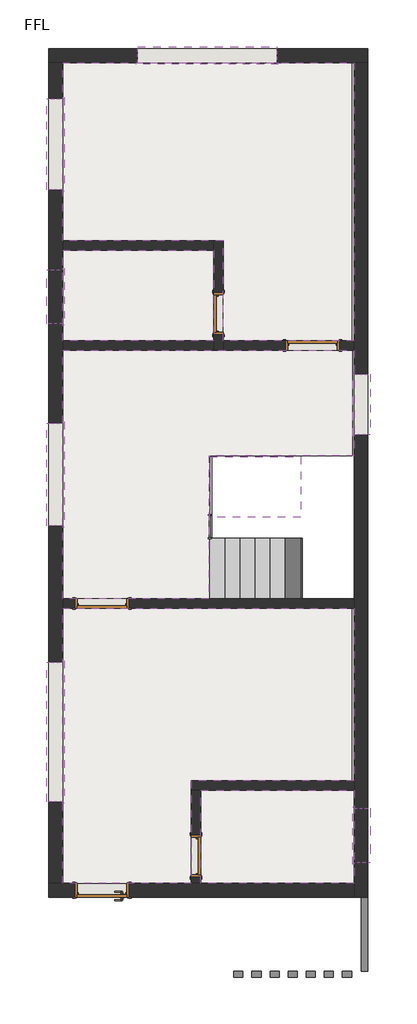
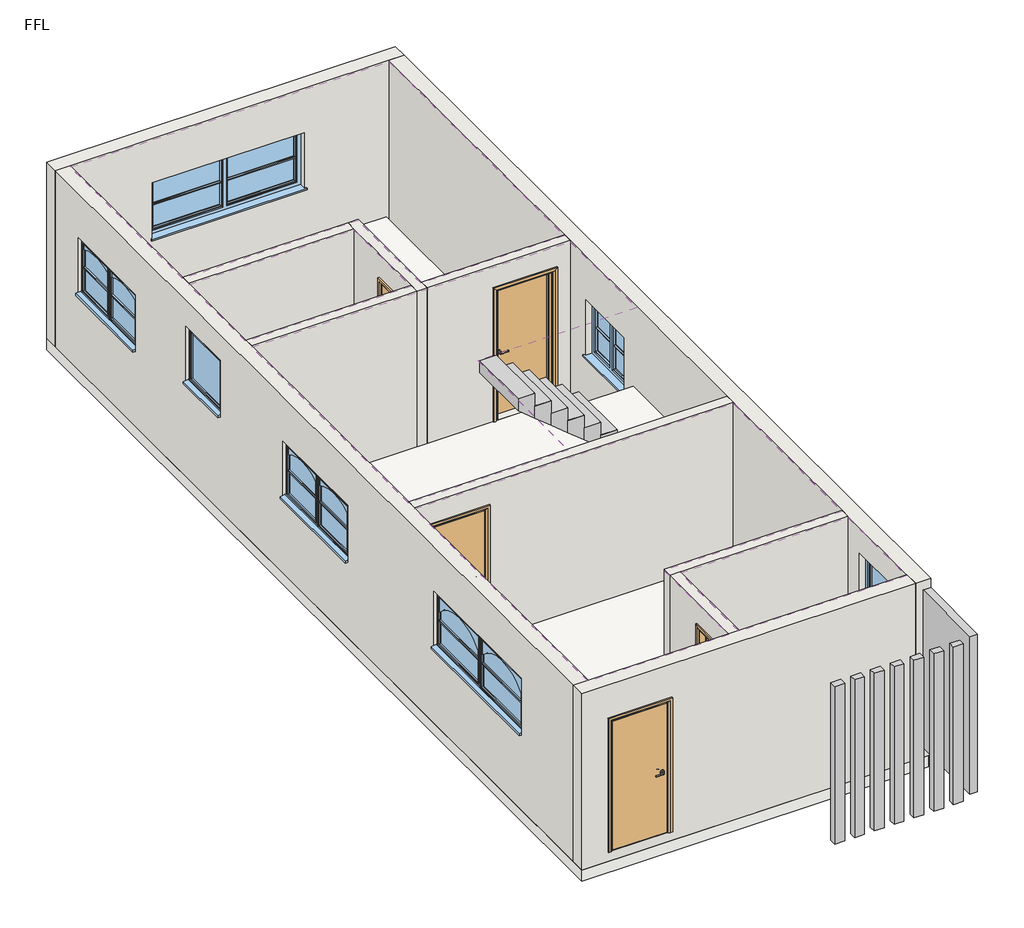
# One storey, incomplete: 11 walls, 7 windows, 6 slabs, 5 coverings, 5 doors, 2 furniture elements, 2 stair flights, 1 railing.
"""IFC4 building model written with IfcOpenShell, lengths in millimetres."""

from ifc_helpers import new_model, si_unit, point, frame, origin, place, context, project, spatial, polyline, ellipse_curve, trimmed, outline, extrude, faceted_brep, transform, mapped, element, save
from ifc_brep_helpers import plane_surface, extruded_surface, advanced_brep
from components import doors_intsgl_1_0_7m_00cad461, doors_intsgl_1_0_7m_20e7f540, doors_intsgl_1_0_9m_7aac3a70, doors_intsgl_1_0_9m_a04e9bb1, casework_1_casework_1_07494d98, casework_3_casework_3_48862e2f, windows_dbl_swept_head_1_m_37dff1ae, windows_dbl_swept_head_1_5_m_7eee1f0c, windows_dbl_swept_head_1_7_m_3b36615c, windows_dbl_swept_head_2_3_m_acbf59cb, windows_sgl_plain_0_9_m_ad1c2cf7

model = new_model("IFC4")

# Units and contexts
model_context = context("Model", 3, world=origin())
ifc_project = project(units=[si_unit("LENGTHUNIT", "METRE", prefix="MILLI")], contexts=[model_context])

# Site, building, storey
site = spatial("IfcSite", under=ifc_project)
building = spatial("IfcBuilding", under=site)
storey = spatial("IfcBuildingStorey", under=building, Name="FFL", Elevation=3000.0)

# Coverings
placement = place(None, origin())
element("IfcCovering", 1, ObjectType="Plain", at=placement, inside=storey, context=model_context, shape_type="SweptSolid", body=[
    extrude(outline(polyline([(-21137.0794706, 13667.7258404), (-16316.1794706, 13667.7258404), (-16316.1794706, 9066.7973913), (-18484.6794706, 9066.7973913), (-18484.6794706, 10719.1973913), (-21137.0794706, 10719.1973913), (-21137.0794706, 13667.7258404)])), frame((0.0, 0.0, 5800.0), z_axis=(0.0, 0.0, 1.0), x_axis=(1.0, 0.0, 0.0)), (0.0, 0.0, 1.0), 57.0),
])
element("IfcCovering", 2, ObjectType="Plain", at=placement, inside=storey, context=model_context, shape_type="SweptSolid", body=[
    extrude(outline(polyline([(-21137.0794706, 9066.7973913), (-21137.0794706, 10566.7973913), (-18637.0794706, 10566.7973913), (-18637.0794706, 9066.7973913), (-21137.0794706, 9066.7973913)])), frame((0.0, 0.0, 5800.0), z_axis=(0.0, 0.0, 1.0), x_axis=(1.0, 0.0, 0.0)), (0.0, 0.0, 1.0), 57.0),
])
element("IfcCovering", 3, ObjectType="Plain", at=placement, inside=storey, context=model_context, shape_type="SweptSolid", body=[
    extrude(outline(polyline([(-16316.1794706, 8914.3973913), (-16316.1794706, 7168.7350753), (-18722.2278737, 7168.7350753), (-18722.2278737, 4801.1258404), (-21137.0794706, 4801.1258404), (-21137.0794706, 8914.3973913), (-18560.8794706, 8914.3973913), (-16316.1794706, 8914.3973913)])), frame((0.0, 0.0, 5800.0), z_axis=(0.0, 0.0, 1.0), x_axis=(1.0, 0.0, 0.0)), (0.0, 0.0, 1.0), 57.0),
])
element("IfcCovering", 4, ObjectType="Plain", at=placement, inside=storey, context=model_context, shape_type="SweptSolid", body=[
    extrude(outline(polyline([(-16316.1794706, 4648.7258404), (-16316.1794706, 1791.1258404), (-19006.6794706, 1791.1258404), (-19006.6794706, 96.3258404), (-21137.0794706, 96.3258404), (-21137.0794706, 4648.7258404), (-16316.1794706, 4648.7258404)])), frame((0.0, 0.0, 5800.0), z_axis=(0.0, 0.0, 1.0), x_axis=(1.0, 0.0, 0.0)), (0.0, 0.0, 1.0), 57.0),
])
element("IfcCovering", 5, ObjectType="Plain", at=placement, inside=storey, context=model_context, shape_type="SweptSolid", body=[
    extrude(outline(polyline([(-18854.2794706, 1638.7258404), (-16316.1794706, 1638.7258404), (-16316.1794706, 96.3258404), (-18854.2794706, 96.3258404), (-18854.2794706, 1638.7258404)])), frame((0.0, 0.0, 5800.0), z_axis=(0.0, 0.0, 1.0), x_axis=(1.0, 0.0, 0.0)), (0.0, 0.0, 1.0), 57.0),
])

# Doors
doors_intsgl_1_0_7m_shape = doors_intsgl_1_0_7m_00cad461(model_context)
element("IfcDoor", 6, ObjectType="Doors_IntSgl_1 : 0.7M", at=placement, inside=storey, context=model_context, shape_type="MappedRepresentation", body=[
    mapped(doors_intsgl_1_0_7m_shape, transform((-18930.4794706, 546.3258404, 3330.0), x_axis=(0.0, -1.0, 0.0), y_axis=(1.0, 0.0, 0.0), z_axis=(0.0, 0.0, 1.0))),
])
doors_intsgl_1_0_7m_2_shape = doors_intsgl_1_0_7m_20e7f540(model_context)
element("IfcDoor", 7, ObjectType="Doors_IntSgl_1 : 0.7M", at=placement, inside=storey, context=model_context, shape_type="MappedRepresentation", body=[
    mapped(doors_intsgl_1_0_7m_2_shape, transform((-18560.8794706, 9516.7973913, 3300.0), x_axis=(0.0, -1.0, 0.0), y_axis=(1.0, 0.0, 0.0), z_axis=(0.0, 0.0, 1.0))),
])
doors_intsgl_1_0_9m_shape = doors_intsgl_1_0_9m_7aac3a70(model_context)
element("IfcDoor", 8, ObjectType="Doors_IntSgl_1 : 0.9M", at=placement, inside=storey, context=model_context, shape_type="MappedRepresentation", body=[
    mapped(doors_intsgl_1_0_9m_shape, transform((-17004.2794706, 8990.5973913, 3330.0), x_axis=(1.0, 0.0, 0.0), y_axis=(0.0, 1.0, 0.0), z_axis=(0.0, 0.0, 1.0))),
])
element("IfcDoor", 9, ObjectType="Doors_IntSgl_1 : 0.9M", at=placement, inside=storey, context=model_context, shape_type="MappedRepresentation", body=[
    mapped(doors_intsgl_1_0_9m_shape, transform((-20487.0794706, 4724.9258404, 3330.0), x_axis=(-1.0, 0.0, 0.0), y_axis=(0.0, -1.0, 0.0), z_axis=(0.0, 0.0, 1.0))),
])
doors_intsgl_1_0_9m_2_shape = doors_intsgl_1_0_9m_a04e9bb1(model_context)
element("IfcDoor", 10, ObjectType="Doors_IntSgl_1 : 0.9M", at=placement, inside=storey, context=model_context, shape_type="MappedRepresentation", body=[
    mapped(doors_intsgl_1_0_9m_2_shape, transform((-20487.0794706, -17.9741596, 3150.0), x_axis=(-1.0, 0.0, 0.0), y_axis=(0.0, -1.0, 0.0), z_axis=(0.0, 0.0, 1.0))),
])

# Furniture
casework_1_casework_1_shape = casework_1_casework_1_07494d98(model_context)
element("IfcFurniture", 11, ObjectType="Casework 1 : Casework 1", at=placement, inside=storey, context=model_context, shape_type="MappedRepresentation", body=[
    mapped(casework_1_casework_1_shape, transform((0.0, 0.0, 0.0), x_axis=(1.0, 0.0, 0.0), y_axis=(0.0, 1.0, 0.0), z_axis=(0.0, 0.0, 1.0))),
])
casework_3_casework_3_shape = casework_3_casework_3_48862e2f(model_context)
element("IfcFurniture", 12, ObjectType="Casework 3 : Casework 3", at=placement, inside=storey, context=model_context, shape_type="MappedRepresentation", body=[
    mapped(casework_3_casework_3_shape, transform((0.0, 0.0, 0.0), x_axis=(1.0, 0.0, 0.0), y_axis=(0.0, 1.0, 0.0), z_axis=(0.0, 0.0, 1.0))),
])

# Railing
element("IfcRailing", 13, ObjectType="Glass_Panel-Bottom_Fill", at=placement, inside=storey, context=model_context, shape_type="SolidModel", body=[
    advanced_brep(
    [(-18745.2702358, 5800.7258404, 4230.0), (-18665.2702358, 5800.7258404, 4230.0), (-18745.2702358, 6188.9258404, 4230.0), (-18665.2702358, 6188.9258404, 4230.0)],
    [
        (0, 1, ellipse_curve(frame((-18705.2702358, 5800.7258404, 4230.0), z_axis=(0.0, -1.0, 0.0), x_axis=(1.0, 0.0, 0.0)), 40.0, 30.0)),
        (1, 0, ellipse_curve(frame((-18705.2702358, 5800.7258404, 4230.0), z_axis=(0.0, -1.0, 0.0), x_axis=(1.0, 0.0, 0.0)), 40.0, 30.0)),
        (2, 3, ellipse_curve(frame((-18705.2702358, 6188.9258404, 4230.0), z_axis=(0.0, 1.0, 0.0), x_axis=(1.0, 0.0, 0.0)), 40.0, 30.0)),
        (3, 2, ellipse_curve(frame((-18705.2702358, 6188.9258404, 4230.0), z_axis=(0.0, 1.0, 0.0), x_axis=(1.0, 0.0, 0.0)), 40.0, 30.0)),
        (0, 2),
        (3, 1),
    ],
    [
        plane_surface(frame((-18705.2702358, 5800.7258404, 4230.0), z_axis=(0.0, -1.0, 0.0), x_axis=(0.0, 0.0, 1.0))),
        plane_surface(frame((-18705.2702358, 6188.9258404, 4230.0), z_axis=(0.0, 1.0, 0.0), x_axis=(0.0, 0.0, 1.0))),
        extruded_surface(trimmed(ellipse_curve(frame((-18705.2702358, 6188.9258404, 4230.0), z_axis=(0.0, -1.0, 0.0), x_axis=(1.0, 0.0, 0.0)), 40.0, 30.0), [point((-18745.2702358, 6188.9258404, 4230.0))], [point((-18665.2702358, 6188.9258404, 4230.0))], True, "CARTESIAN"), (0.0, -388.1999999999998, 0.0), 388.1999999999998),
        extruded_surface(trimmed(ellipse_curve(frame((-18705.2702358, 6188.9258404, 4230.0), z_axis=(0.0, -1.0, 0.0), x_axis=(1.0, 0.0, 0.0)), 40.0, 30.0), [point((-18665.2702358, 6188.9258404, 4230.0))], [point((-18745.2702358, 6188.9258404, 4230.0))], True, "CARTESIAN"), (0.0, -388.1999999999998, 0.0), 388.1999999999998),
    ],
    [
        (0, [[1, 2]]),
        (1, [[3, 4]]),
        (2, [[-1, 5, -4, 6]]),
        (3, [[-2, -6, -3, -5]]),
    ],
),
    extrude(outline(polyline([(-18695.8794706, 5800.7258404), (-18715.8794706, 5800.7258404), (-18715.8794706, 6188.9258404), (-18695.8794706, 6188.9258404), (-18695.8794706, 5800.7258404)])), frame((0.0, 0.0, 4110.0), z_axis=(0.0, 0.0, 1.0), x_axis=(1.0, 0.0, 0.0)), (0.0, 0.0, 1.0), 20.0),
    extrude(outline(polyline([(-18695.8794706, 5800.7258404), (-18715.8794706, 5800.7258404), (-18715.8794706, 6188.9258404), (-18695.8794706, 6188.9258404), (-18695.8794706, 5800.7258404)])), frame((0.0, 0.0, 4010.0), z_axis=(0.0, 0.0, 1.0), x_axis=(1.0, 0.0, 0.0)), (0.0, 0.0, 1.0), 20.0),
    extrude(outline(polyline([(-18730.8794706, 6180.9258404), (-18730.8794706, 6192.9258404), (-18680.8794706, 6192.9258404), (-18680.8794706, 6180.9258404), (-18730.8794706, 6180.9258404)])), frame((0.0, 0.0, 3330.0), z_axis=(0.0, 0.0, 1.0), x_axis=(1.0, 0.0, 0.0)), (0.0, 0.0, 1.0), 870.0),
    extrude(outline(polyline([(-18730.8794706, 5796.7258404), (-18730.8794706, 5808.7258404), (-18680.8794706, 5808.7258404), (-18680.8794706, 5796.7258404), (-18730.8794706, 5796.7258404)])), frame((0.0, 0.0, 3330.0), z_axis=(0.0, 0.0, 1.0), x_axis=(1.0, 0.0, 0.0)), (0.0, 0.0, 1.0), 870.0),
])

# Slabs
element("IfcSlab", 14, ObjectType="200mm_Thickness", at=placement, inside=storey, context=model_context, shape_type="SolidModel", body=[
    faceted_brep([(-17201.8794706, 5801.1258404, 4574.0), (-17201.8794706, 4801.1258404, 4574.0), (-16959.9361063, 4801.1258404, 4574.0), (-16381.8794706, 4801.1258404, 4574.0), (-16381.8794706, 7153.5258404, 4574.0), (-17193.8228349, 7153.5258404, 4574.0), (-17201.8794706, 7153.5258404, 4574.0), (-17201.8794706, 6153.5258404, 4574.0), (-17201.8794706, 5801.1258404, 4374.0), (-17201.8794706, 5801.1258404, 4370.4285714), (-17201.8794706, 5801.1258404, 4176.9889748), (-17201.8794706, 4801.1258404, 4176.9889748), (-17201.8794706, 4801.1258404, 4370.4285714), (-16959.9361063, 4801.1258404, 4374.0), (-16381.8794706, 4801.1258404, 4374.0), (-16381.8794706, 7153.5258404, 4374.0), (-17193.8228349, 7153.5258404, 4374.0), (-17201.8794706, 7153.5258404, 4380.5604034), (-17201.8794706, 6153.5258404, 4380.5604034), (-17201.8794706, 6153.5258404, 4374.0), (-17193.8228349, 6153.5258404, 4374.0), (-16959.9361063, 5801.1258404, 4374.0)], [[[0, 1, 2, 3, 4, 5, 6, 7]], [[1, 0, 8, 9, 10, 11, 12]], [[1, 12, 11, 13, 14, 3, 2]], [[4, 3, 14, 15]], [[4, 15, 16, 17, 6, 5]], [[7, 6, 17, 18]], [[0, 7, 18, 19, 8]], [[19, 20, 16, 15, 14, 13, 21, 8]], [[20, 19, 18]], [[21, 13, 11, 10]], [[8, 21, 10, 9]], [[16, 20, 18, 17]]]),
    extrude(outline(polyline([(-17201.8794706, 5801.1258404), (-17201.8794706, 6153.5258404), (-17201.8794706, 7153.5258404), (-16381.8794706, 7153.5258404), (-16381.8794706, 4801.1258404), (-17201.8794706, 4801.1258404), (-17201.8794706, 5801.1258404)])), frame((0.0, 0.0, 4574.0), z_axis=(0.0, 0.0, 1.0), x_axis=(1.0, 0.0, 0.0)), (0.0, 0.0, 1.0), 1.0),
])
element("IfcSlab", 15, ObjectType="BEDROOM FLOOR", at=placement, inside=storey, context=model_context, shape_type="SweptSolid", body=[
    extrude(outline(polyline([(-21137.0794706, 13667.7258404), (-16354.2794706, 13667.7258404), (-16354.2794706, 9066.7973913), (-18484.6794706, 9066.7973913), (-18484.6794706, 10719.1973913), (-21137.0794706, 10719.1973913), (-21137.0794706, 13667.7258404)])), frame((0.0, 0.0, 3180.0), z_axis=(0.0, 0.0, 1.0), x_axis=(1.0, 0.0, 0.0)), (0.0, 0.0, 1.0), 150.0),
    extrude(outline(polyline([(-19006.6794706, 96.3258404), (-21137.0794706, 96.3258404), (-21137.0794706, 4648.7258404), (-18589.4794706, 4648.7258404), (-16354.2794706, 4648.7258404), (-16354.2794706, 1791.1258404), (-19006.6794706, 1791.1258404), (-19006.6794706, 96.3258404)])), frame((0.0, 0.0, 3180.0), z_axis=(0.0, 0.0, 1.0), x_axis=(1.0, 0.0, 0.0)), (0.0, 0.0, 1.0), 150.0),
])
element("IfcSlab", 16, ObjectType="FAMILY LOUNGE", at=placement, inside=storey, context=model_context, shape_type="SweptSolid", body=[
    extrude(outline(polyline([(-18701.8794706, 4801.1258404), (-21137.0794706, 4801.1258404), (-21137.0794706, 8914.3973913), (-16351.8794706, 8914.3973913), (-16351.8794706, 7168.7613597), (-18701.8794706, 7168.7613597), (-18701.8794706, 4801.1258404)])), frame((0.0, 0.0, 3180.0), z_axis=(0.0, 0.0, 1.0), x_axis=(1.0, 0.0, 0.0)), (0.0, 0.0, 1.0), 150.0),
])
element("IfcSlab", 17, ObjectType="SLAB", at=placement, inside=storey, context=model_context, shape_type="SweptSolid", body=[
    extrude(outline(polyline([(-16125.6794706, 13896.3258404), (-16125.6794706, -132.2741596), (-21365.6794706, -132.2741596), (-21365.6794706, 13896.3258404), (-16125.6794706, 13896.3258404)]), holes=[polyline([(-16316.1794706, 7168.7350753), (-18663.7794706, 7168.7350753), (-18663.7794706, 4801.1258404), (-16316.1794706, 4801.1258404), (-16316.1794706, 7168.7350753)])]), frame((0.0, 0.0, 2820.0), z_axis=(0.0, 0.0, 1.0), x_axis=(1.0, 0.0, 0.0)), (0.0, 0.0, 1.0), 180.0),
])
element("IfcSlab", 18, ObjectType="TOILET FLOOR", at=placement, inside=storey, context=model_context, shape_type="SweptSolid", body=[
    extrude(outline(polyline([(-18637.0794706, 10566.7973913), (-18637.0794706, 9066.7973913), (-21137.0794706, 9066.7973913), (-21137.0794706, 10566.7973913), (-18637.0794706, 10566.7973913)])), frame((0.0, 0.0, 3000.0), z_axis=(0.0, 0.0, 1.0), x_axis=(1.0, 0.0, 0.0)), (0.0, 0.0, 1.0), 300.0),
])
element("IfcSlab", 19, ObjectType="TOILET FLOOR", at=placement, inside=storey, context=model_context, shape_type="SweptSolid", body=[
    extrude(outline(polyline([(-16316.1794706, 1638.7258404), (-16316.1794706, 96.3258404), (-18854.2794706, 96.3258404), (-18854.2794706, 1638.7258404), (-16316.1794706, 1638.7258404)])), frame((0.0, 0.0, 3000.0), z_axis=(0.0, 0.0, 1.0), x_axis=(1.0, 0.0, 0.0)), (0.0, 0.0, 1.0), 300.0),
])

# Stair flights
element("IfcStairFlight", 20, ObjectType="1mm_Tread-150mm_Depth", at=placement, inside=storey, context=model_context, shape_type="SolidModel", body=[
    faceted_brep([(-18451.8794706, 5801.1258404, 3352.5714286), (-18701.8794706, 5801.1258404, 3352.5714286), (-18701.8794706, 4801.1258404, 3352.5714286), (-18451.8794706, 4801.1258404, 3352.5714286), (-18451.8794706, 5801.1258404, 3159.1318319), (-18463.0940011, 5801.1258404, 3150.0), (-18701.8794706, 5801.1258404, 3150.0), (-18701.8794706, 4801.1258404, 3150.0), (-18463.0940011, 4801.1258404, 3150.0), (-18451.8794706, 4801.1258404, 3159.1318319), (-18201.8794706, 5801.1258404, 3556.1428571), (-18451.8794706, 5801.1258404, 3556.1428571), (-18451.8794706, 4801.1258404, 3556.1428571), (-18201.8794706, 4801.1258404, 3556.1428571), (-18201.8794706, 5801.1258404, 3362.7032605), (-18201.8794706, 4801.1258404, 3362.7032605), (-17951.8794706, 5801.1258404, 3759.7142857), (-18201.8794706, 5801.1258404, 3759.7142857), (-18201.8794706, 4801.1258404, 3759.7142857), (-17951.8794706, 4801.1258404, 3759.7142857), (-17951.8794706, 5801.1258404, 3566.2746891), (-17951.8794706, 4801.1258404, 3566.2746891), (-17701.8794706, 5801.1258404, 3963.2857143), (-17951.8794706, 5801.1258404, 3963.2857143), (-17951.8794706, 4801.1258404, 3963.2857143), (-17701.8794706, 4801.1258404, 3963.2857143), (-17701.8794706, 5801.1258404, 3769.8461176), (-17701.8794706, 4801.1258404, 3769.8461176), (-17451.8794706, 5801.1258404, 4166.8571429), (-17701.8794706, 5801.1258404, 4166.8571429), (-17701.8794706, 4801.1258404, 4166.8571429), (-17451.8794706, 4801.1258404, 4166.8571429), (-17451.8794706, 5801.1258404, 3973.4175462), (-17451.8794706, 4801.1258404, 3973.4175462), (-17201.8794706, 5801.1258404, 4370.4285714), (-17451.8794706, 5801.1258404, 4370.4285714), (-17451.8794706, 4801.1258404, 4370.4285714), (-17201.8794706, 4801.1258404, 4370.4285714), (-17201.8794706, 5801.1258404, 4176.9889748), (-17201.8794706, 4801.1258404, 4176.9889748)], [[[0, 1, 2, 3]], [[1, 0, 4, 5, 6]], [[2, 1, 6, 7]], [[3, 2, 7, 8, 9]], [[10, 11, 12, 13]], [[11, 10, 14, 4, 0]], [[0, 3, 12, 11]], [[13, 12, 3, 9, 15]], [[16, 17, 18, 19]], [[17, 16, 20, 14, 10]], [[10, 13, 18, 17]], [[19, 18, 13, 15, 21]], [[22, 23, 24, 25]], [[23, 22, 26, 20, 16]], [[16, 19, 24, 23]], [[25, 24, 19, 21, 27]], [[28, 29, 30, 31]], [[29, 28, 32, 26, 22]], [[22, 25, 30, 29]], [[31, 30, 25, 27, 33]], [[34, 35, 36, 37]], [[35, 34, 38, 32, 28]], [[28, 31, 36, 35]], [[37, 36, 31, 33, 39]], [[34, 37, 39, 38]], [[7, 6, 5, 8]], [[8, 5, 4, 14, 20, 26, 32, 38, 39, 33, 27, 21, 15, 9]]]),
    extrude(outline(polyline([(-18451.8794706, 5801.1258404), (-18451.8794706, 4801.1258404), (-18701.8794706, 4801.1258404), (-18701.8794706, 5801.1258404), (-18451.8794706, 5801.1258404)])), frame((0.0, 0.0, 3352.5714286), z_axis=(0.0, 0.0, 1.0), x_axis=(1.0, 0.0, 0.0)), (0.0, 0.0, 1.0), 1.0),
    extrude(outline(polyline([(-18201.8794706, 5801.1258404), (-18201.8794706, 4801.1258404), (-18451.8794706, 4801.1258404), (-18451.8794706, 5801.1258404), (-18201.8794706, 5801.1258404)])), frame((0.0, 0.0, 3556.1428571), z_axis=(0.0, 0.0, 1.0), x_axis=(1.0, 0.0, 0.0)), (0.0, 0.0, 1.0), 1.0),
    extrude(outline(polyline([(-17951.8794706, 5801.1258404), (-17951.8794706, 4801.1258404), (-18201.8794706, 4801.1258404), (-18201.8794706, 5801.1258404), (-17951.8794706, 5801.1258404)])), frame((0.0, 0.0, 3759.7142857), z_axis=(0.0, 0.0, 1.0), x_axis=(1.0, 0.0, 0.0)), (0.0, 0.0, 1.0), 1.0),
    extrude(outline(polyline([(-17701.8794706, 5801.1258404), (-17701.8794706, 4801.1258404), (-17951.8794706, 4801.1258404), (-17951.8794706, 5801.1258404), (-17701.8794706, 5801.1258404)])), frame((0.0, 0.0, 3963.2857143), z_axis=(0.0, 0.0, 1.0), x_axis=(1.0, 0.0, 0.0)), (0.0, 0.0, 1.0), 1.0),
    extrude(outline(polyline([(-17451.8794706, 5801.1258404), (-17451.8794706, 4801.1258404), (-17701.8794706, 4801.1258404), (-17701.8794706, 5801.1258404), (-17451.8794706, 5801.1258404)])), frame((0.0, 0.0, 4166.8571429), z_axis=(0.0, 0.0, 1.0), x_axis=(1.0, 0.0, 0.0)), (0.0, 0.0, 1.0), 1.0),
    extrude(outline(polyline([(-17201.8794706, 5801.1258404), (-17201.8794706, 4801.1258404), (-17451.8794706, 4801.1258404), (-17451.8794706, 5801.1258404), (-17201.8794706, 5801.1258404)])), frame((0.0, 0.0, 4370.4285714), z_axis=(0.0, 0.0, 1.0), x_axis=(1.0, 0.0, 0.0)), (0.0, 0.0, 1.0), 1.0),
])
element("IfcStairFlight", 21, ObjectType="1mm_Tread-150mm_Depth", at=placement, inside=storey, context=model_context, shape_type="SolidModel", body=[
    faceted_brep([(-17451.8794706, 6153.5258404, 4777.5714286), (-17201.8794706, 6153.5258404, 4777.5714286), (-17201.8794706, 7153.5258404, 4777.5714286), (-17451.8794706, 7153.5258404, 4777.5714286), (-17451.8794706, 6153.5258404, 4584.1318319), (-17201.8794706, 6153.5258404, 4380.5604034), (-17201.8794706, 7153.5258404, 4380.5604034), (-17201.8794706, 7153.5258404, 4574.0), (-17451.8794706, 7153.5258404, 4584.1318319), (-17701.8794706, 6153.5258404, 4981.1428571), (-17451.8794706, 6153.5258404, 4981.1428571), (-17451.8794706, 7153.5258404, 4981.1428571), (-17701.8794706, 7153.5258404, 4981.1428571), (-17701.8794706, 6153.5258404, 4787.7032605), (-17701.8794706, 7153.5258404, 4787.7032605), (-17951.8794706, 6153.5258404, 5184.7142857), (-17701.8794706, 6153.5258404, 5184.7142857), (-17701.8794706, 7153.5258404, 5184.7142857), (-17951.8794706, 7153.5258404, 5184.7142857), (-17951.8794706, 6153.5258404, 4991.2746891), (-17951.8794706, 7153.5258404, 4991.2746891), (-18201.8794706, 6153.5258404, 5388.2857143), (-17951.8794706, 6153.5258404, 5388.2857143), (-17951.8794706, 7153.5258404, 5388.2857143), (-18201.8794706, 7153.5258404, 5388.2857143), (-18201.8794706, 6153.5258404, 5194.8461176), (-18201.8794706, 7153.5258404, 5194.8461176), (-18451.8794706, 6153.5258404, 5591.8571429), (-18201.8794706, 6153.5258404, 5591.8571429), (-18201.8794706, 7153.5258404, 5591.8571429), (-18451.8794706, 7153.5258404, 5591.8571429), (-18451.8794706, 6153.5258404, 5398.4175462), (-18451.8794706, 7153.5258404, 5398.4175462), (-18701.8794706, 6153.5258404, 5795.4285714), (-18451.8794706, 6153.5258404, 5795.4285714), (-18451.8794706, 7153.5258404, 5795.4285714), (-18701.8794706, 7153.5258404, 5795.4285714), (-18701.8794706, 6153.5258404, 5601.9889748), (-18701.8794706, 7153.5258404, 5601.9889748)], [[[0, 1, 2, 3]], [[1, 0, 4, 5]], [[2, 1, 5, 6, 7]], [[3, 2, 7, 6, 8]], [[9, 10, 11, 12]], [[10, 9, 13, 4, 0]], [[11, 10, 0, 3]], [[12, 11, 3, 8, 14]], [[15, 16, 17, 18]], [[16, 15, 19, 13, 9]], [[17, 16, 9, 12]], [[18, 17, 12, 14, 20]], [[21, 22, 23, 24]], [[22, 21, 25, 19, 15]], [[23, 22, 15, 18]], [[24, 23, 18, 20, 26]], [[27, 28, 29, 30]], [[28, 27, 31, 25, 21]], [[29, 28, 21, 24]], [[30, 29, 24, 26, 32]], [[33, 34, 35, 36]], [[34, 33, 37, 31, 27]], [[35, 34, 27, 30]], [[36, 35, 30, 32, 38]], [[33, 36, 38, 37]], [[5, 4, 13, 19, 25, 31, 37, 38, 32, 26, 20, 14, 8, 6]]]),
    extrude(outline(polyline([(-17451.8794706, 6153.5258404), (-17451.8794706, 7153.5258404), (-17201.8794706, 7153.5258404), (-17201.8794706, 6153.5258404), (-17451.8794706, 6153.5258404)])), frame((0.0, 0.0, 4777.5714286), z_axis=(0.0, 0.0, 1.0), x_axis=(1.0, 0.0, 0.0)), (0.0, 0.0, 1.0), 1.0),
    extrude(outline(polyline([(-17701.8794706, 6153.5258404), (-17701.8794706, 7153.5258404), (-17451.8794706, 7153.5258404), (-17451.8794706, 6153.5258404), (-17701.8794706, 6153.5258404)])), frame((0.0, 0.0, 4981.1428571), z_axis=(0.0, 0.0, 1.0), x_axis=(1.0, 0.0, 0.0)), (0.0, 0.0, 1.0), 1.0),
    extrude(outline(polyline([(-17951.8794706, 6153.5258404), (-17951.8794706, 7153.5258404), (-17701.8794706, 7153.5258404), (-17701.8794706, 6153.5258404), (-17951.8794706, 6153.5258404)])), frame((0.0, 0.0, 5184.7142857), z_axis=(0.0, 0.0, 1.0), x_axis=(1.0, 0.0, 0.0)), (0.0, 0.0, 1.0), 1.0),
    extrude(outline(polyline([(-18201.8794706, 6153.5258404), (-18201.8794706, 7153.5258404), (-17951.8794706, 7153.5258404), (-17951.8794706, 6153.5258404), (-18201.8794706, 6153.5258404)])), frame((0.0, 0.0, 5388.2857143), z_axis=(0.0, 0.0, 1.0), x_axis=(1.0, 0.0, 0.0)), (0.0, 0.0, 1.0), 1.0),
    extrude(outline(polyline([(-18451.8794706, 6153.5258404), (-18451.8794706, 7153.5258404), (-18201.8794706, 7153.5258404), (-18201.8794706, 6153.5258404), (-18451.8794706, 6153.5258404)])), frame((0.0, 0.0, 5591.8571429), z_axis=(0.0, 0.0, 1.0), x_axis=(1.0, 0.0, 0.0)), (0.0, 0.0, 1.0), 1.0),
    extrude(outline(polyline([(-18701.8794706, 6153.5258404), (-18701.8794706, 7153.5258404), (-18451.8794706, 7153.5258404), (-18451.8794706, 6153.5258404), (-18701.8794706, 6153.5258404)])), frame((0.0, 0.0, 5795.4285714), z_axis=(0.0, 0.0, 1.0), x_axis=(1.0, 0.0, 0.0)), (0.0, 0.0, 1.0), 1.0),
])

# Walls
element("IfcWall", 22, at=placement, inside=storey, context=model_context, shape_type="SweptSolid", body=[
    extrude(outline(polyline([(3000.0, -18484.6794706), (3000.0, -16316.1794706), (5820.0, -16316.1794706), (5820.0, -18484.6794706), (3000.0, -18484.6794706)]), holes=[polyline([(5440.0, -16554.2794706), (3330.0, -16554.2794706), (3330.0, -17454.2794706), (5440.0, -17454.2794706), (5440.0, -16554.2794706)])]), frame((0.0, 8914.3973913, 0.0), z_axis=(0.0, 1.0, 0.0), x_axis=(0.0, 0.0, 1.0)), (0.0, 0.0, 1.0), 152.4),
])
element("IfcWall", 23, at=placement, inside=storey, context=model_context, shape_type="SweptSolid", body=[
    extrude(outline(polyline([(3000.0, -21137.0794706), (3000.0, -16316.1794706), (5820.0, -16316.1794706), (5820.0, -21137.0794706), (3000.0, -21137.0794706)]), holes=[polyline([(3330.0, -20937.0794706), (5440.0, -20937.0794706), (5440.0, -20037.0794706), (3330.0, -20037.0794706), (3330.0, -20937.0794706)])]), frame((0.0, 4648.7258404, 0.0), z_axis=(0.0, 1.0, 0.0), x_axis=(0.0, 0.0, 1.0)), (0.0, 0.0, 1.0), 152.4),
])
element("IfcWall", 24, at=placement, inside=storey, context=model_context, shape_type="Brep", body=[
    faceted_brep([(-18637.0794706, 10719.1973913, 3000.0), (-18637.0794706, 10566.7973913, 3000.0), (-18637.0794706, 9066.7973913, 3000.0), (-18637.0794706, 8914.3973913, 3000.0), (-18637.0794706, 8914.3973913, 5820.0), (-18637.0794706, 9066.7973913, 5820.0), (-18637.0794706, 10566.7973913, 5820.0), (-18637.0794706, 10719.1973913, 5820.0), (-18637.0794706, 9166.7973913, 5410.0), (-18637.0794706, 9166.7973913, 3300.0), (-18637.0794706, 9866.7973913, 3300.0), (-18637.0794706, 9866.7973913, 5410.0), (-18484.6794706, 8914.3973913, 3000.0), (-18484.6794706, 9066.7973913, 3000.0), (-18484.6794706, 10719.1973913, 3000.0), (-18484.6794706, 10719.1973913, 5820.0), (-18484.6794706, 9066.7973913, 5820.0), (-18484.6794706, 8914.3973913, 5820.0), (-18484.6794706, 9166.7973913, 3300.0), (-18484.6794706, 9166.7973913, 5410.0), (-18484.6794706, 9866.7973913, 5410.0), (-18484.6794706, 9866.7973913, 3300.0)], [[[0, 1, 2, 3, 4, 5, 6, 7], [8, 9, 10, 11]], [[12, 13, 14, 15, 16, 17], [18, 19, 20, 21]], [[3, 2, 1, 0, 14, 13, 12]], [[7, 6, 5, 4, 17, 16, 15]], [[4, 3, 12, 17]], [[0, 7, 15, 14]], [[18, 9, 8, 19]], [[19, 8, 11, 20]], [[20, 11, 10, 21]], [[9, 18, 21, 10]]]),
])
element("IfcWall", 25, at=placement, inside=storey, context=model_context, shape_type="SweptSolid", body=[
    extrude(outline(polyline([(-21137.0794706, 9066.7973913), (-18637.0794706, 9066.7973913), (-18637.0794706, 8914.3973913), (-21137.0794706, 8914.3973913), (-21137.0794706, 9066.7973913)])), frame((0.0, 0.0, 3000.0), z_axis=(0.0, 0.0, 1.0), x_axis=(1.0, 0.0, 0.0)), (0.0, 0.0, 1.0), 2820.0),
])
element("IfcWall", 26, at=placement, inside=storey, context=model_context, shape_type="SweptSolid", body=[
    extrude(outline(polyline([(-21137.0794706, 10719.1973913), (-18637.0794706, 10719.1973913), (-18637.0794706, 10566.7973913), (-21137.0794706, 10566.7973913), (-21137.0794706, 10719.1973913)])), frame((0.0, 0.0, 3000.0), z_axis=(0.0, 0.0, 1.0), x_axis=(1.0, 0.0, 0.0)), (0.0, 0.0, 1.0), 2820.0),
])
element("IfcWall", 27, at=placement, inside=storey, context=model_context, shape_type="Brep", body=[
    faceted_brep([(-16316.1794706, 1791.1258404, 3000.0), (-19006.6794706, 1791.1258404, 3000.0), (-19006.6794706, 1791.1258404, 5820.0), (-16316.1794706, 1791.1258404, 5820.0), (-16316.1794706, 1638.7258404, 3000.0), (-16316.1794706, 1638.7258404, 5820.0), (-18854.2794706, 1638.7258404, 5820.0), (-19006.6794706, 1638.7258404, 5820.0), (-19006.6794706, 1638.7258404, 3000.0), (-18854.2794706, 1638.7258404, 3000.0)], [[[0, 1, 2, 3]], [[4, 5, 6, 7, 8, 9]], [[1, 0, 4, 9, 8]], [[3, 2, 7, 6, 5]], [[0, 3, 5, 4]], [[2, 1, 8, 7]]]),
])
element("IfcWall", 28, at=placement, inside=storey, context=model_context, shape_type="SweptSolid", body=[
    extrude(outline(polyline([(1638.7258404, 3000.0), (96.3258404, 3000.0), (96.3258404, 5820.0), (1638.7258404, 5820.0), (1638.7258404, 3000.0)]), holes=[polyline([(196.3258404, 5440.0), (196.3258404, 3330.0), (896.3258404, 3330.0), (896.3258404, 5440.0), (196.3258404, 5440.0)])]), frame((-19006.6794706, 0.0, 0.0), z_axis=(1.0, 0.0, 0.0), x_axis=(0.0, 1.0, 0.0)), (0.0, 0.0, 1.0), 152.4),
])
element("IfcWall", 29, ObjectType="EX WALL", at=placement, inside=storey, context=model_context, shape_type="Brep", body=[
    faceted_brep([(-21365.6794706, 13667.7258404, 3000.0), (-21137.0794706, 13667.7258404, 3000.0), (-16316.1794706, 13667.7258404, 3000.0), (-16087.5794706, 13667.7258404, 3000.0), (-16087.5794706, 13667.7258404, 5820.0), (-16316.1794706, 13667.7258404, 5820.0), (-21137.0794706, 13667.7258404, 5820.0), (-21365.6794706, 13667.7258404, 5820.0), (-19895.6794706, 13667.7258404, 5110.0), (-17595.6794706, 13667.7258404, 5110.0), (-17595.6794706, 13667.7258404, 4200.0), (-19895.6794706, 13667.7258404, 4200.0), (-21365.6794706, 13896.3258404, 3000.0), (-21365.6794706, 13896.3258404, 5820.0), (-16087.5794706, 13896.3258404, 5820.0), (-16087.5794706, 13896.3258404, 3000.0), (-19895.6794706, 13896.3258404, 5110.0), (-19895.6794706, 13896.3258404, 4200.0), (-17595.6794706, 13896.3258404, 4200.0), (-17595.6794706, 13896.3258404, 5110.0)], [[[0, 1, 2, 3, 4, 5, 6, 7], [8, 9, 10, 11]], [[12, 13, 14, 15], [16, 17, 18, 19]], [[3, 2, 1, 0, 12, 15]], [[7, 6, 5, 4, 14, 13]], [[4, 3, 15, 14]], [[0, 7, 13, 12]], [[17, 16, 8, 11]], [[18, 17, 11, 10]], [[19, 18, 10, 9]], [[16, 19, 9, 8]]]),
])
element("IfcWall", 30, ObjectType="EX WALL", at=placement, inside=storey, context=model_context, shape_type="Brep", body=[
    faceted_brep([(-16316.1794706, 13667.7258404, 3000.0), (-16316.1794706, 9066.7973913, 3000.0), (-16316.1794706, 8914.3973913, 3000.0), (-16316.1794706, 4801.1258404, 3000.0), (-16316.1794706, 4648.7258404, 3000.0), (-16316.1794706, 1791.1258404, 3000.0), (-16316.1794706, 1638.7258404, 3000.0), (-16316.1794706, 96.3258404, 3000.0), (-16316.1794706, -132.2741596, 3000.0), (-16316.1794706, -132.2741596, 5820.0), (-16316.1794706, 96.3258404, 5820.0), (-16316.1794706, 1638.7258404, 5820.0), (-16316.1794706, 1791.1258404, 5820.0), (-16316.1794706, 4648.7258404, 5820.0), (-16316.1794706, 4801.1258404, 5820.0), (-16316.1794706, 8914.3973913, 5820.0), (-16316.1794706, 9066.7973913, 5820.0), (-16316.1794706, 13667.7258404, 5820.0), (-16316.1794706, 8514.3973913, 5110.0), (-16316.1794706, 7514.3973913, 5110.0), (-16316.1794706, 7514.3973913, 4200.0), (-16316.1794706, 8514.3973913, 4200.0), (-16316.1794706, 1338.7258404, 5410.0), (-16316.1794706, 438.7258404, 5410.0), (-16316.1794706, 438.7258404, 4500.0), (-16316.1794706, 1338.7258404, 4500.0), (-16087.5794706, 13667.7258404, 3000.0), (-16087.5794706, 13667.7258404, 5820.0), (-16087.5794706, -132.2741596, 5820.0), (-16087.5794706, -132.2741596, 3000.0), (-16087.5794706, 8514.3973913, 5110.0), (-16087.5794706, 8514.3973913, 4200.0), (-16087.5794706, 7514.3973913, 4200.0), (-16087.5794706, 7514.3973913, 5110.0), (-16087.5794706, 1338.7258404, 5410.0), (-16087.5794706, 1338.7258404, 4500.0), (-16087.5794706, 438.7258404, 4500.0), (-16087.5794706, 438.7258404, 5410.0)], [[[0, 1, 2, 3, 4, 5, 6, 7, 8, 9, 10, 11, 12, 13, 14, 15, 16, 17], [18, 19, 20, 21], [22, 23, 24, 25]], [[26, 27, 28, 29], [30, 31, 32, 33], [34, 35, 36, 37]], [[8, 7, 6, 5, 4, 3, 2, 1, 0, 26, 29]], [[17, 16, 15, 14, 13, 12, 11, 10, 9, 28, 27]], [[0, 17, 27, 26]], [[9, 8, 29, 28]], [[31, 30, 18, 21]], [[32, 31, 21, 20]], [[33, 32, 20, 19]], [[30, 33, 19, 18]], [[35, 34, 22, 25]], [[36, 35, 25, 24]], [[37, 36, 24, 23]], [[34, 37, 23, 22]]]),
])
element("IfcWall", 31, ObjectType="EX WALL", at=placement, inside=storey, context=model_context, shape_type="Brep", body=[
    faceted_brep([(-16316.1794706, 96.3258404, 3000.0), (-18854.2794706, 96.3258404, 3000.0), (-19006.6794706, 96.3258404, 3000.0), (-21137.0794706, 96.3258404, 3000.0), (-21365.6794706, 96.3258404, 3000.0), (-21365.6794706, 96.3258404, 5820.0), (-21137.0794706, 96.3258404, 5820.0), (-19006.6794706, 96.3258404, 5820.0), (-18854.2794706, 96.3258404, 5820.0), (-16316.1794706, 96.3258404, 5820.0), (-20937.0794706, 96.3258404, 5260.0), (-20937.0794706, 96.3258404, 3150.0), (-20037.0794706, 96.3258404, 3150.0), (-20037.0794706, 96.3258404, 5260.0), (-21365.6794706, -132.2741596, 3000.0), (-16316.1794706, -132.2741596, 3000.0), (-16316.1794706, -132.2741596, 5820.0), (-21365.6794706, -132.2741596, 5820.0), (-20937.0794706, -132.2741596, 3150.0), (-20937.0794706, -132.2741596, 5260.0), (-20037.0794706, -132.2741596, 5260.0), (-20037.0794706, -132.2741596, 3150.0)], [[[0, 1, 2, 3, 4, 5, 6, 7, 8, 9], [10, 11, 12, 13]], [[14, 15, 16, 17], [18, 19, 20, 21]], [[4, 3, 2, 1, 0, 15, 14]], [[9, 8, 7, 6, 5, 17, 16]], [[0, 9, 16, 15]], [[5, 4, 14, 17]], [[18, 11, 10, 19]], [[19, 10, 13, 20]], [[20, 13, 12, 21]], [[11, 18, 21, 12]]]),
])
element("IfcWall", 32, ObjectType="EX WALL", at=placement, inside=storey, context=model_context, shape_type="Brep", body=[
    faceted_brep([(-21137.0794706, 96.3258404, 3000.0), (-21137.0794706, 4648.7258404, 3000.0), (-21137.0794706, 4801.1258404, 3000.0), (-21137.0794706, 8914.3973913, 3000.0), (-21137.0794706, 9066.7973913, 3000.0), (-21137.0794706, 10566.7973913, 3000.0), (-21137.0794706, 10719.1973913, 3000.0), (-21137.0794706, 13667.7258404, 3000.0), (-21137.0794706, 13667.7258404, 5820.0), (-21137.0794706, 10719.1973913, 5820.0), (-21137.0794706, 10566.7973913, 5820.0), (-21137.0794706, 9066.7973913, 5820.0), (-21137.0794706, 8914.3973913, 5820.0), (-21137.0794706, 4801.1258404, 5820.0), (-21137.0794706, 4648.7258404, 5820.0), (-21137.0794706, 96.3258404, 5820.0), (-21137.0794706, 6007.7616159, 5110.0), (-21137.0794706, 7707.7616159, 5110.0), (-21137.0794706, 7707.7616159, 4200.0), (-21137.0794706, 6007.7616159, 4200.0), (-21137.0794706, 11567.7258404, 5110.0), (-21137.0794706, 13067.7258404, 5110.0), (-21137.0794706, 13067.7258404, 4200.0), (-21137.0794706, 11567.7258404, 4200.0), (-21137.0794706, 1448.7258404, 5110.0), (-21137.0794706, 3748.7258404, 5110.0), (-21137.0794706, 3748.7258404, 4200.0), (-21137.0794706, 1448.7258404, 4200.0), (-21137.0794706, 9346.7973913, 5410.0), (-21137.0794706, 10246.7973913, 5410.0), (-21137.0794706, 10246.7973913, 4500.0), (-21137.0794706, 9346.7973913, 4500.0), (-21365.6794706, 96.3258404, 3000.0), (-21365.6794706, 96.3258404, 5820.0), (-21365.6794706, 13667.7258404, 5820.0), (-21365.6794706, 13667.7258404, 3000.0), (-21365.6794706, 6007.7616159, 5110.0), (-21365.6794706, 6007.7616159, 4200.0), (-21365.6794706, 7707.7616159, 4200.0), (-21365.6794706, 7707.7616159, 5110.0), (-21365.6794706, 11567.7258404, 5110.0), (-21365.6794706, 11567.7258404, 4200.0), (-21365.6794706, 13067.7258404, 4200.0), (-21365.6794706, 13067.7258404, 5110.0), (-21365.6794706, 1448.7258404, 5110.0), (-21365.6794706, 1448.7258404, 4200.0), (-21365.6794706, 3748.7258404, 4200.0), (-21365.6794706, 3748.7258404, 5110.0), (-21365.6794706, 9346.7973913, 5410.0), (-21365.6794706, 9346.7973913, 4500.0), (-21365.6794706, 10246.7973913, 4500.0), (-21365.6794706, 10246.7973913, 5410.0)], [[[0, 1, 2, 3, 4, 5, 6, 7, 8, 9, 10, 11, 12, 13, 14, 15], [16, 17, 18, 19], [20, 21, 22, 23], [24, 25, 26, 27], [28, 29, 30, 31]], [[32, 33, 34, 35], [36, 37, 38, 39], [40, 41, 42, 43], [44, 45, 46, 47], [48, 49, 50, 51]], [[7, 6, 5, 4, 3, 2, 1, 0, 32, 35]], [[15, 14, 13, 12, 11, 10, 9, 8, 34, 33]], [[8, 7, 35, 34]], [[0, 15, 33, 32]], [[37, 36, 16, 19]], [[38, 37, 19, 18]], [[39, 38, 18, 17]], [[36, 39, 17, 16]], [[41, 40, 20, 23]], [[42, 41, 23, 22]], [[43, 42, 22, 21]], [[40, 43, 21, 20]], [[45, 44, 24, 27]], [[46, 45, 27, 26]], [[47, 46, 26, 25]], [[44, 47, 25, 24]], [[49, 48, 28, 31]], [[50, 49, 31, 30]], [[51, 50, 30, 29]], [[48, 51, 29, 28]]]),
])

# Windows
windows_dbl_swept_head_1_m_shape = windows_dbl_swept_head_1_m_37dff1ae(model_context)
element("IfcWindow", 33, ObjectType="Windows_Dbl_Swept_Head : 1 M", at=placement, inside=storey, context=model_context, shape_type="MappedRepresentation", body=[
    mapped(windows_dbl_swept_head_1_m_shape, transform((-16210.3360384, 7729.3973913, 3000.0), x_axis=(0.0, -1.0, 0.0), y_axis=(1.0, 0.0, 0.0), z_axis=(0.0, 0.0, 1.0))),
])
windows_dbl_swept_head_1_5_m_shape = windows_dbl_swept_head_1_5_m_7eee1f0c(model_context)
element("IfcWindow", 34, ObjectType="Windows_Dbl_Swept_Head : 1.5 M", at=placement, inside=storey, context=model_context, shape_type="MappedRepresentation", body=[
    mapped(windows_dbl_swept_head_1_5_m_shape, transform((-21242.9229028, 12602.7258404, 3000.0), x_axis=(0.0, 1.0, 0.0), y_axis=(-1.0, 0.0, 0.0), z_axis=(0.0, 0.0, 1.0))),
])
windows_dbl_swept_head_1_7_m_shape = windows_dbl_swept_head_1_7_m_3b36615c(model_context)
element("IfcWindow", 35, ObjectType="Windows_Dbl_Swept_Head : 1.7 M", at=placement, inside=storey, context=model_context, shape_type="MappedRepresentation", body=[
    mapped(windows_dbl_swept_head_1_7_m_shape, transform((-21242.9229028, 7142.7616159, 3000.0), x_axis=(0.0, 1.0, 0.0), y_axis=(-1.0, 0.0, 0.0), z_axis=(0.0, 0.0, 1.0))),
])
windows_dbl_swept_head_2_3_m_shape = windows_dbl_swept_head_2_3_m_acbf59cb(model_context)
element("IfcWindow", 36, ObjectType="Windows_Dbl_Swept_Head : 2.3 M", at=placement, inside=storey, context=model_context, shape_type="MappedRepresentation", body=[
    mapped(windows_dbl_swept_head_2_3_m_shape, transform((-18460.6794706, 13773.5692726, 3000.0), x_axis=(1.0, 0.0, 0.0), y_axis=(0.0, 1.0, 0.0), z_axis=(0.0, 0.0, 1.0))),
])
element("IfcWindow", 37, ObjectType="Windows_Dbl_Swept_Head : 2.3 M", at=placement, inside=storey, context=model_context, shape_type="MappedRepresentation", body=[
    mapped(windows_dbl_swept_head_2_3_m_shape, transform((-21242.9229028, 2883.7258404, 3000.0), x_axis=(0.0, 1.0, 0.0), y_axis=(-1.0, 0.0, 0.0), z_axis=(0.0, 0.0, 1.0))),
])
windows_sgl_plain_0_9_m_shape = windows_sgl_plain_0_9_m_ad1c2cf7(model_context)
element("IfcWindow", 38, ObjectType="Windows_Sgl_Plain : 0.9 M", at=placement, inside=storey, context=model_context, shape_type="MappedRepresentation", body=[
    mapped(windows_sgl_plain_0_9_m_shape, transform((-21242.9229028, 9796.7973913, 3300.0), x_axis=(0.0, 1.0, 0.0), y_axis=(-1.0, 0.0, 0.0), z_axis=(0.0, 0.0, 1.0))),
])
element("IfcWindow", 39, ObjectType="Windows_Sgl_Plain : 0.9 M", at=placement, inside=storey, context=model_context, shape_type="MappedRepresentation", body=[
    mapped(windows_sgl_plain_0_9_m_shape, transform((-16210.3360384, 888.7258404, 3300.0), x_axis=(0.0, -1.0, 0.0), y_axis=(1.0, 0.0, 0.0), z_axis=(0.0, 0.0, 1.0))),
])

save(model, "model.ifc")

# Revit data of these elements
# Type "Plain"
#   Keynote = "K40"
#   built-in parameter 1002203 = 1 (stored number, unit not read)
#   built-in parameter 1002202 = 1 (stored number, unit not read)
#   Layers, outside or top first: 0.045 m "Metal Stud Layer" (function 1); 0.012 m "Gypsum Wall Board" (function 1)
# Type "Doors_IntSgl_1 : 0.7M"
#   Type Mark = "58"
#   Type Comments = "Internal Single"
#   Operation = "SingleSwingRight"
#   Construction Type Id = "MDOOR"
#   Manufacturer = "Revit"
#   Keynote = "L20"
#   Description = "Internal Single Door"
#   Analytic Construction = "Metal"
#   UnderCut = 0.008 m
#   Tolerance = 0.002 m
#   Thickness = 0.038 m
#   Structural Tolerance = 0.008 m
#   StopDepth = 0.032 m
#   Stop Thickness = 0.019 m
#   Rough Width = 0.7 m
#   Rough Height = 2.11 m
#   Height to Top Lock Rail = 1.0 m
#   Heat Transfer Coefficient (U) = 3.7021 W/(m²·K)
#   Handle Z Distance = 1.0 m
#   Handle X Distance = 0.075 m
#   Frame Thickness = 0.032 m
#   Door Panel Width = 0.616 m
#   Door Panel Thickness = 0.038 m
#   Door Panel Offset = 0.0 m
#   Height = 2.11 m
#   Width = 0.7 m
#   Door Panel Height = 2.06 m
#   Architrave Setback = 0.005 m
#   Vis - Ironmongery = yes
#   Define Thermal Properties by = 1
#   Material Ironmongery = Door - Handle
#   Material Frame = Door - Frame/Mullion
#   Material Door = Door - Panel
#   Material Architrave = Door - Architrave
#   Visual Light Transmittance = 0
#   Solar Heat Gain Coefficient = 0
#   Function = (empty or 0)
#   Wall Closure = (empty or 0)
# Type "Doors_IntSgl_1 : 0.9M"
#   Type Mark = "57"
#   Type Comments = "Internal Single"
#   Operation = "SingleSwingRight"
#   Construction Type Id = "MDOOR"
#   Manufacturer = "Revit"
#   Keynote = "L20"
#   Description = "Internal Single Door"
#   Analytic Construction = "Metal"
#   UnderCut = 0.008 m
#   Tolerance = 0.002 m
#   Thickness = 0.038 m
#   Structural Tolerance = 0.008 m
#   StopDepth = 0.032 m
#   Stop Thickness = 0.019 m
#   Rough Width = 0.9 m
#   Rough Height = 2.11 m
#   Height to Top Lock Rail = 1.0 m
#   Heat Transfer Coefficient (U) = 3.7021 W/(m²·K)
#   Handle Z Distance = 1.0 m
#   Handle X Distance = 0.075 m
#   Frame Thickness = 0.032 m
#   Door Panel Width = 0.816 m
#   Door Panel Thickness = 0.038 m
#   Door Panel Offset = 0.0 m
#   Height = 2.11 m
#   Width = 0.9 m
#   Door Panel Height = 2.06 m
#   Architrave Setback = 0.005 m
#   Vis - Ironmongery = yes
#   Define Thermal Properties by = 1
#   Material Ironmongery = Door - Handle
#   Material Frame = Door - Frame/Mullion
#   Material Door = Door - Panel
#   Material Architrave = Door - Architrave
#   Visual Light Transmittance = 0
#   Solar Heat Gain Coefficient = 0
#   Function = (empty or 0)
#   Wall Closure = (empty or 0)
# Type "Glass_Panel-Bottom_Fill"
#   built-in parameter 1008612 = 0.019685 (stored number, unit not read)
#   built-in parameter 1008611 = 0.019685 (stored number, unit not read)
#   built-in parameter 1008609 = 0.902231 (stored number, unit not read)
#   built-in parameter 1008604 = 0.19685 (stored number, unit not read)
#   built-in parameter 1008603 = 0.164042 (stored number, unit not read)
#   Railing Height = 0.9 m
#   built-in parameter 1008630 = 2
#   built-in parameter 1008610 = 2
# Type "BEDROOM FLOOR"
#   Function = 0
#   Layers, outside or top first: 0.022 m "Wood Sheathing, Chipboard" (function 5); 0.128 m "Structure, Timber Joist/Rafter Layer" (function 1)
# Type "FAMILY LOUNGE"
#   Function = 0
#   Layers, outside or top first: 0.022 m "Wood Sheathing, Chipboard" (function 5); 0.128 m "Structure, Timber Joist/Rafter Layer" (function 1)
# Type "SLAB"
#   Layers, outside or top first: 0.18 m "Concrete, Cast In Situ" (function 1)
# Type "TOILET FLOOR"
#   Function = 0
#   Layers, outside or top first: 0.05 m "Wood Sheathing, Chipboard" (function 5); 0.25 m "Structure, Timber Joist/Rafter Layer" (function 1)
# Type
#   Keynote = "F10"
#   Layers, outside or top first: 0.1524 m "WHITE BOARD" (function 1)
# Type "EX WALL"
#   Keynote = "F10"
#   Layers, outside or top first: 0.2286 m "WHITE BOARD" (function 1)
# Type "Windows_Dbl_Swept_Head : 1 M"
#   Type Mark = "67"
#   Operation = "DoublePanelVertical"
#   Construction Type Id = "GSP4R"
#   Manufacturer = "Revit"
#   Keynote = "L10"
#   Analytic Construction = "1/8 in Pilkington single glazing"
#   Wrap Layers (Ext) from Ext = 0.1025 m
#   Wrap Layers (Int) from Ext = 0.1775 m
#   Window Board Projection = 0.025 m
#   Window Board Extension = 0.025 m
#   Visual Light Transmittance = 0.9
#   Solar Heat Gain Coefficient = 0.78
#   Rough Width = 1.0 m
#   Rough Height = 0.91 m
#   Radius - Swept Head = 0.7 m
#   Height = 0.91 m
#   Width = 1.0 m
#   Heat Transfer Coefficient (U) = 3.6886 W/(m²·K)
#   Glazing Thickness = 0.024 m
#   FrameOffset - External = 0.05 m
#   Frame Depth = 0.065 m
#   Default Head Height = 2.11 m
#   Cill Depth = 0.0875 m
#   Cavity Closer Width = 0.05 m
#   Cavity Closer Offset from Ext = 0.1025 m
#   Cavity Closer Depth = 0.085 m
#   Vis - Cavity Closers = yes
#   Define Thermal Properties by = 1
#   Material Trim = Window Frame
#   Material Glass = Glass
#   Material Frame = Window Frame
#   Wall Closure = (empty or 0)
# Type "Windows_Dbl_Swept_Head : 1.5 M"
#   Type Mark = "70"
#   Operation = "DoublePanelVertical"
#   Construction Type Id = "GSP4R"
#   Manufacturer = "Revit"
#   Keynote = "L10"
#   Analytic Construction = "1/8 in Pilkington single glazing"
#   Wrap Layers (Ext) from Ext = 0.1025 m
#   Wrap Layers (Int) from Ext = 0.1775 m
#   Window Board Projection = 0.025 m
#   Window Board Extension = 0.025 m
#   Visual Light Transmittance = 0.9
#   Solar Heat Gain Coefficient = 0.78
#   Rough Width = 1.5 m
#   Rough Height = 0.91 m
#   Radius - Swept Head = 0.7 m
#   Height = 0.91 m
#   Width = 1.5 m
#   Heat Transfer Coefficient (U) = 3.6886 W/(m²·K)
#   Glazing Thickness = 0.024 m
#   FrameOffset - External = 0.05 m
#   Frame Depth = 0.065 m
#   Default Head Height = 2.11 m
#   Cill Depth = 0.0875 m
#   Cavity Closer Width = 0.05 m
#   Cavity Closer Offset from Ext = 0.1025 m
#   Cavity Closer Depth = 0.085 m
#   Vis - Cavity Closers = yes
#   Define Thermal Properties by = 1
#   Material Trim = Window Frame
#   Material Glass = Glass
#   Material Frame = Window Frame
#   Wall Closure = (empty or 0)
# Type "Windows_Dbl_Swept_Head : 1.7 M"
#   Type Mark = "68"
#   Operation = "DoublePanelVertical"
#   Construction Type Id = "GSP4R"
#   Manufacturer = "Revit"
#   Keynote = "L10"
#   Analytic Construction = "1/8 in Pilkington single glazing"
#   Wrap Layers (Ext) from Ext = 0.1025 m
#   Wrap Layers (Int) from Ext = 0.1775 m
#   Window Board Projection = 0.025 m
#   Window Board Extension = 0.025 m
#   Visual Light Transmittance = 0.9
#   Solar Heat Gain Coefficient = 0.78
#   Rough Width = 1.7 m
#   Rough Height = 0.91 m
#   Radius - Swept Head = 0.7 m
#   Height = 0.91 m
#   Width = 1.7 m
#   Heat Transfer Coefficient (U) = 3.6886 W/(m²·K)
#   Glazing Thickness = 0.024 m
#   FrameOffset - External = 0.05 m
#   Frame Depth = 0.065 m
#   Default Head Height = 2.11 m
#   Cill Depth = 0.0875 m
#   Cavity Closer Width = 0.05 m
#   Cavity Closer Offset from Ext = 0.1025 m
#   Cavity Closer Depth = 0.085 m
#   Vis - Cavity Closers = yes
#   Define Thermal Properties by = 1
#   Material Trim = Window Frame
#   Material Glass = Glass
#   Material Frame = Window Frame
#   Wall Closure = (empty or 0)
# Type "Windows_Dbl_Swept_Head : 2.3 M"
#   Type Mark = "69"
#   Operation = "DoublePanelVertical"
#   Construction Type Id = "GSP4R"
#   Manufacturer = "Revit"
#   Keynote = "L10"
#   Analytic Construction = "1/8 in Pilkington single glazing"
#   Wrap Layers (Ext) from Ext = 0.1025 m
#   Wrap Layers (Int) from Ext = 0.1775 m
#   Window Board Projection = 0.025 m
#   Window Board Extension = 0.025 m
#   Visual Light Transmittance = 0.9
#   Solar Heat Gain Coefficient = 0.78
#   Rough Width = 2.3 m
#   Rough Height = 0.91 m
#   Radius - Swept Head = 0.7 m
#   Height = 0.91 m
#   Width = 2.3 m
#   Heat Transfer Coefficient (U) = 3.6886 W/(m²·K)
#   Glazing Thickness = 0.024 m
#   FrameOffset - External = 0.05 m
#   Frame Depth = 0.065 m
#   Default Head Height = 2.11 m
#   Cill Depth = 0.0875 m
#   Cavity Closer Width = 0.05 m
#   Cavity Closer Offset from Ext = 0.1025 m
#   Cavity Closer Depth = 0.085 m
#   Vis - Cavity Closers = yes
#   Define Thermal Properties by = 1
#   Material Trim = Window Frame
#   Material Glass = Glass
#   Material Frame = Window Frame
#   Wall Closure = (empty or 0)
# Type "Windows_Sgl_Plain : 0.9 M"
#   Type Mark = "59"
#   Operation = "SinglePanel"
#   Construction Type Id = "SGL"
#   Manufacturer = "Revit"
#   Keynote = "L10"
#   Analytic Construction = "Large single-glazed windows"
#   Wrap Layers (Ext) from Ext = 0.1025 m
#   Wrap Layers (Int) from Ext = 0.1775 m
#   Window Board Projection = 0.025 m
#   Window Board Extension = 0.025 m
#   Visual Light Transmittance = 0.9
#   Solar Heat Gain Coefficient = 0.86
#   Rough Width = 0.9 m
#   Rough Height = 0.91 m
#   Height = 0.91 m
#   Width = 0.9 m
#   Heat Transfer Coefficient (U) = 5.5617 W/(m²·K)
#   Glazing Thickness = 0.024 m
#   FrameOffset - External = 0.05 m
#   Frame Depth = 0.065 m
#   Default Head Height = 2.11 m
#   Cill Depth = 0.0875 m
#   Cavity Closer Width = 0.05 m
#   Cavity Closer Offset from Ext = 0.1025 m
#   Cavity Closer Depth = 0.085 m
#   Vis - Cavity Closers = yes
#   Define Thermal Properties by = 1
#   Material Trim = Window Frame
#   Material Glass = Glass
#   Material Frame = Window Frame
#   Wall Closure = (empty or 0)
# Elements 1, 2, 3, 4, 5 (IfcCovering, "Plain")
#   Height Offset From Level = 2.8 m
#   Phase Created = New Construction
#   Materials on its faces: "Gypsum Wall Board", "Metal Stud Layer"
# Elements 6, 7 (IfcDoor, "Doors_IntSgl_1 : 0.7M")
#   Phase Created = New Construction
#   Materials on its faces: "Door - Architrave", "Door - Handle", "Door - Frame/Mullion", "Door - Panel"
# Elements 8, 9, 10 (IfcDoor, "Doors_IntSgl_1 : 0.9M")
#   Phase Created = New Construction
#   Materials on its faces: "Door - Architrave", "Door - Handle", "Door - Frame/Mullion", "Door - Panel"
# Element 11 (IfcFurniture, "Casework 1 : Casework 1")
#   Phase Created = New Construction
# Element 12 (IfcFurniture, "Casework 3 : Casework 3")
#   Phase Created = New Construction
# Element 13 (IfcRailing, "Glass_Panel-Bottom_Fill")
#   built-in parameter 1008621 = 1.08268 (stored number, unit not read)
#   Phase Created = New Construction
#   Materials on its faces: "Metal - Stainless Steel,Polished"
# Element 14 (IfcSlab, "200mm_Thickness")
#   Phase Created = New Construction
#   Materials on its faces: "Concrete, Cast-in-Place gray"
# Element 15 (IfcSlab, "BEDROOM FLOOR")
#   built-in parameter 1001955 = 1.5708 (stored number, unit not read)
#   Height Offset From Level = 0.33 m
#   Phase Created = New Construction
#   Materials on its faces: "Structure, Timber Joist/Rafter Layer", "Wood Sheathing, Chipboard"
# Element 16 (IfcSlab, "FAMILY LOUNGE")
#   Height Offset From Level = 0.33 m
#   Phase Created = New Construction
#   Materials on its faces: "Structure, Timber Joist/Rafter Layer", "Wood Sheathing, Chipboard"
# Element 17 (IfcSlab, "SLAB")
#   Height Offset From Level = 0.0 m
#   built-in parameter 1001954 = 1
#   Phase Created = New Construction
#   Materials on its faces: "Concrete, Cast In Situ"
# Elements 18, 19 (IfcSlab, "TOILET FLOOR")
#   Height Offset From Level = 0.3 m
#   Phase Created = New Construction
#   Materials on its faces: "Structure, Timber Joist/Rafter Layer", "Wood Sheathing, Chipboard"
# Elements 20, 21 (IfcStairFlight, "1mm_Tread-150mm_Depth")
#   Phase Created = New Construction
#   Materials on its faces: "Concrete, Cast-in-Place gray"
# Elements 22, 23, 24, 25, 26, 27, 28 (IfcWall)
#   Top Offset = -0.18 m
#   Base Offset = 0.0 m
#   wall height = 2.82 m
#   Phase Created = New Construction
#   Base Constraint = FFL
#   Top Constraint = TL
#   Materials on its faces: "WHITE BOARD"
# Elements 29, 30, 31, 32 (IfcWall, "EX WALL")
#   Top Offset = -0.18 m
#   Base Offset = 0.0 m
#   wall height = 2.82 m
#   Phase Created = New Construction
#   Base Constraint = FFL
#   Top Constraint = TL
#   Materials on its faces: "WHITE BOARD"
# Element 33 (IfcWindow, "Windows_Dbl_Swept_Head : 1 M")
#   Mark = "9"
#   Phase Created = New Construction
#   Materials on its faces: "Window Frame", "Glass"
# Element 34 (IfcWindow, "Windows_Dbl_Swept_Head : 1.5 M")
#   Mark = "8"
#   Phase Created = New Construction
#   Materials on its faces: "Window Frame", "Glass"
# Element 35 (IfcWindow, "Windows_Dbl_Swept_Head : 1.7 M")
#   Mark = "6"
#   Phase Created = New Construction
#   Materials on its faces: "Window Frame", "Glass"
# Element 36 (IfcWindow, "Windows_Dbl_Swept_Head : 2.3 M")
#   Mark = "7"
#   Phase Created = New Construction
#   Materials on its faces: "Window Frame", "Glass"
# Element 37 (IfcWindow, "Windows_Dbl_Swept_Head : 2.3 M")
#   Mark = "10"
#   Phase Created = New Construction
#   Materials on its faces: "Window Frame", "Glass"
# Element 38 (IfcWindow, "Windows_Sgl_Plain : 0.9 M")
#   Mark = "12"
#   Phase Created = New Construction
#   Materials on its faces: "Window Frame", "Glass"
# Element 39 (IfcWindow, "Windows_Sgl_Plain : 0.9 M")
#   Mark = "13"
#   Phase Created = New Construction
#   Materials on its faces: "Window Frame", "Glass"
# Materials
#   "Metal Stud Layer": class "Metal", colour RGB 127 127 127, transparency 0, Description = "Light gauge steel framing, thermal air layer", Cost = 0
#   "Gypsum Wall Board": class "Generic", colour RGB 249 249 249, transparency 0, Description = "Gypsum Wall Board", Cost = 0
#   "Door - Handle": colour RGB 0 0 0, transparency 0, Keynote = "P21", Cost = 0
#   "Door - Frame/Mullion": class "Wood", colour RGB 212 179 113, transparency 0, Keynote = "L20", Cost = 0
#   "Door - Panel": class "Wood", colour RGB 210 159 95, transparency 0, Keynote = "L20", Cost = 0
#   "Door - Architrave": class "Wood", colour RGB 154 90 5, transparency 0, Keynote = "P20", Cost = 0
#   "Wood Sheathing, Chipboard": class "Wood", colour RGB 127 127 127, transparency 0, Description = "Particleboard sheathing", Cost = 0
#   "Structure, Timber Joist/Rafter Layer": class "Wood", colour RGB 127 127 127, transparency 0, Description = "Timber framing, thermal airspace", Cost = 0
#   "Concrete, Cast In Situ": class "Concrete", colour RGB 192 192 192, transparency 0, Description = "physical material", Cost = 0
#   "WHITE BOARD": class "Generic", colour RGB 249 249 249, transparency 0, Description = "Plaster", Cost = 0
#   "Window Frame": colour RGB 249 249 249, transparency 0, Keynote = "L10", Cost = 0
#   "Glass": class "Glass", colour RGB 0 128 192, transparency 0.9, Description = "Soda Lime Glass", Cost = 0
#   "Metal - Stainless Steel,Polished": class "Metal", colour RGB 236 239 239, transparency 0, Cost = 0
#   "Concrete, Cast-in-Place gray": class "Concrete", colour RGB 192 192 192, transparency 0, Description = "Cast-in-place concrete", Cost = 0
